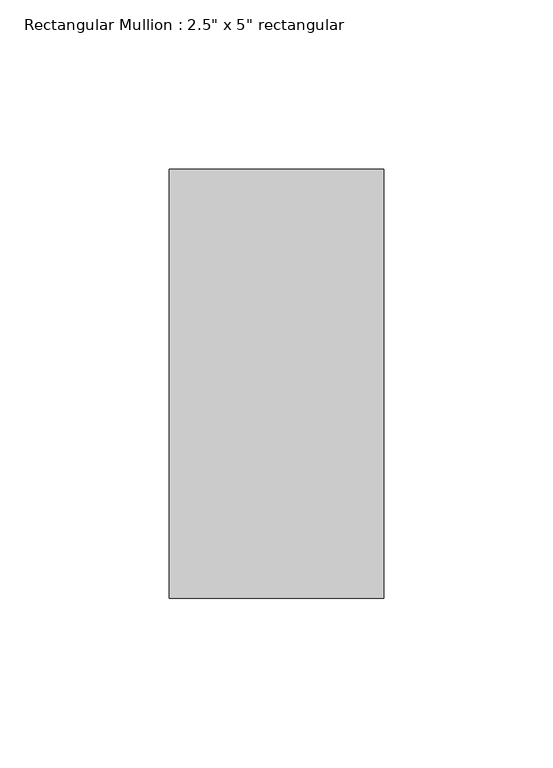
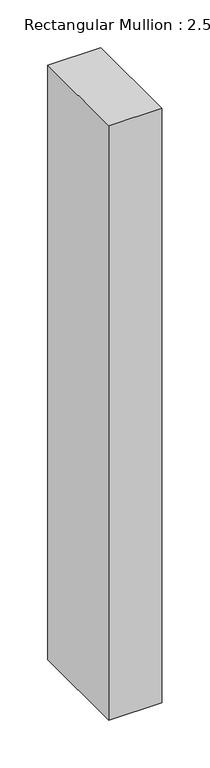
"""IFC4 building model written with IfcOpenShell, lengths in millimetres: member geometry."""

from ifc_helpers import new_model, si_unit, frame, origin, place, context, project, spatial, polyline, outline, extrude, source, transform, mapped, element, save


def member_eb7364f1(model_context):
    return source(origin(), model_context, "Body", "SweptSolid", [
        extrude(outline(polyline([(31.75, 63.5), (31.75, -63.5), (-31.75, -63.5), (-31.75, 63.5), (31.75, 63.5)])), frame((0.0, 0.0, -756.3361093), z_axis=(0.0, 0.0, 1.0), x_axis=(1.0, 0.0, 0.0)), (0.0, 0.0, 1.0), 756.3361093),
    ])


if __name__ == "__main__":
    model = new_model("IFC4")
    model_context = context("Model", 3, world=origin())
    ifc_project = project(units=[si_unit("LENGTHUNIT", "METRE", prefix="MILLI")], contexts=[model_context])
    site = spatial("IfcSite", under=ifc_project)
    building = spatial("IfcBuilding", under=site)
    placement = place(None, origin())
    member_shape = member_eb7364f1(model_context)
    element("IfcMember", 1, ObjectType="Rectangular Mullion : 2.5\" x 5\" rectangular", at=placement, inside=building, context=model_context, shape_type="MappedRepresentation", body=[
        mapped(member_shape, transform((0.0, 0.0, 0.0), x_axis=(1.0, 0.0, 0.0), y_axis=(0.0, 1.0, 0.0), z_axis=(0.0, 0.0, 1.0))),
    ])
    save(model, "model.ifc")

# Revit data of these elements
# Type "Rectangular Mullion : 2.5\" x 5\" rectangular"
#   built-in parameter 1007304 = 0.416667 (stored number, unit not read)
#   built-in parameter 1007301 = 0.104167 (stored number, unit not read)
#   built-in parameter 1007300 = 0.104167 (stored number, unit not read)
# Element 1 (IfcMember, "Rectangular Mullion : 2.5\" x 5\" rectangular")
#   Materials on its faces: "Aluminum"
# Materials
#   "Aluminum": class "Metal", colour RGB 247 247 247, transparency 0, Description = "Aluminum 6061", Cost = 0
